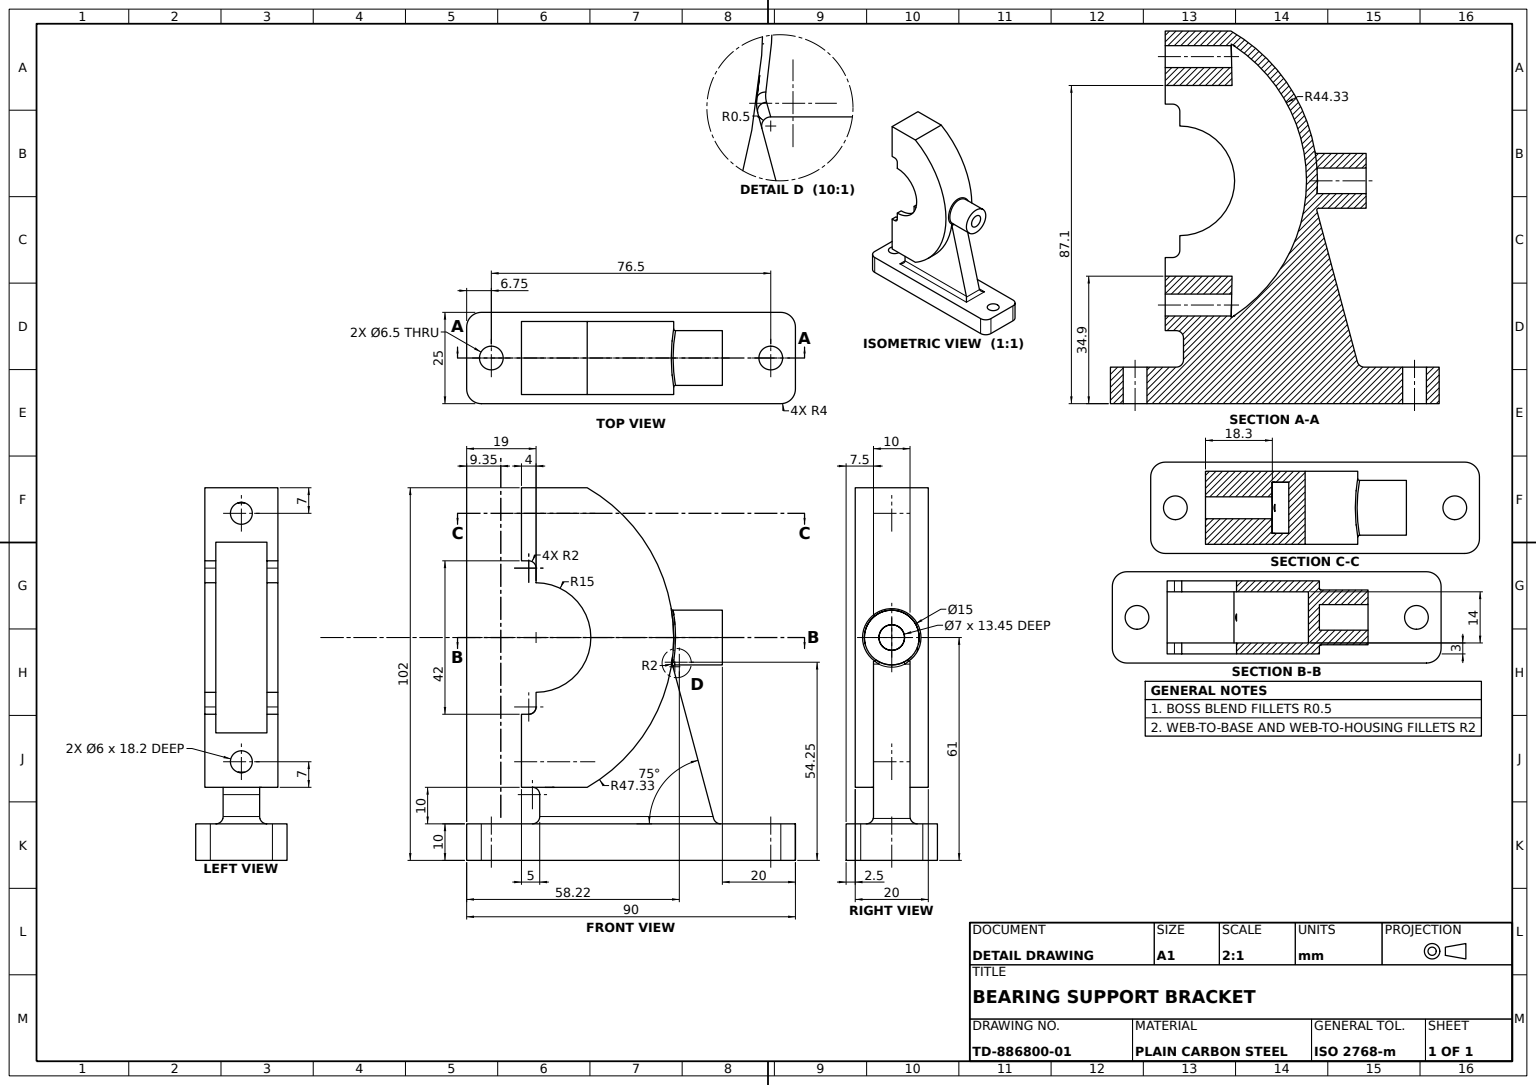
from build123d import *

# Parameters (mm, degrees)
BASE_PLATE_DEPTH              = 10
MOUNTING_HOLES_SKETCH_R       = 3.25
MOUNTING_HOLES_2X_6_5_DEPTH   = 10
UPRIGHT_WEB_SKETCH_W          = 48
UPRIGHT_WEB_SKETCH_H          = 12
UPRIGHT_WEB_DEPTH             = 30
UPRIGHT_WEB_TAPER             = 3
HOUSING_HALF_DEPTH            = 3
HOUSING_ARC_CUT_DEPTH         = 20
WEB_RELIEF_CUT_SKETCH_W       = 13.847905122
WEB_RELIEF_CUT_SKETCH_H       = 28.94973959
WEB_RELIEF_CUT_DEPTH          = 60
HOUSING_LUG_DEPTH             = 14
HOUSING_FLANGE_DEPTH          = 3
HOUSING_RIB_DEPTH             = 20
HOUSING_RELIEF_CUT_DEPTH      = 15
HOUSING_BODY_DEPTH            = 10
FILL_BLOCK_SKETCH_W           = 51.167533007
FILL_BLOCK_SKETCH_H           = 15.02058519
FILL_BLOCK_DEPTH              = 10
BEARING_SEAT_NOTCH_SKETCH_W   = 20.979401449
BEARING_SEAT_NOTCH_SKETCH_H   = 6.47797526
BEARING_SEAT_NOTCH_DEPTH      = 10
BASE_TO_HOUSING_FILLET_R2_R   = 2
SPLIT_BOLT_HOLES_SKETCH_R     = 3
SPLIT_BOLT_HOLES_DEPTH        = 19
FLANGE_FILLET_R2_R            = 2
HOUSING_EDGE_FILLET_R2_R      = 2
GREASE_NIPPLE_BOSS_SKETCH_R   = 7.5
GREASE_NIPPLE_BOSS_SKETCH_R_2 = 3.5
GREASE_NIPPLE_BOSS_DEPTH      = 15
GREASE_BOSS_FILLET_R0_5_R     = 0.5


with BuildPart() as part:
    # Base Plate Sketch → Base Plate (new body)
    with BuildSketch(Plane(origin=(0, 0, 0), x_dir=(1, 0, 0), z_dir=(0, 1, 0))):
        with BuildLine():
            Line((-41, 12.5), (41, 12.5))
            ThreePointArc((41, 12.5), (43.828427125, 11.328427125), (45, 8.5))
            Line((45, 8.5), (45, -8.5))
            ThreePointArc((45, -8.5), (43.828427125, -11.328427125), (41, -12.5))
            Line((41, -12.5), (-41, -12.5))
            ThreePointArc((-41, -12.5), (-43.828427125, -11.328427125), (-45, -8.5))
            Line((-45, -8.5), (-45, 8.5))
            ThreePointArc((-45, 8.5), (-43.828427125, 11.328427125), (-41, 12.5))
        make_face()
    extrude(amount=BASE_PLATE_DEPTH)

    # Mounting Holes Sketch → Mounting Holes 2xØ6.5 (cut)
    with BuildSketch(Plane(origin=(0, 10, 0), x_dir=(1, 0, 0), z_dir=(0, 1, 0))):
        with Locations(Location((-38.25, 0, 0), (0, 0, 270))):
            Circle(MOUNTING_HOLES_SKETCH_R)
        with Locations(Location((38.25, 0, 0), (0, 0, 270))):
            Circle(MOUNTING_HOLES_SKETCH_R)
    extrude(amount=-MOUNTING_HOLES_2X_6_5_DEPTH, mode=Mode.SUBTRACT)

    # Upright Web Sketch → Upright Web (add)
    with BuildSketch(Plane(origin=(0, 10, 0), x_dir=(1, 0, 0), z_dir=(0, 1, 0))):
        Rectangle(UPRIGHT_WEB_SKETCH_W, UPRIGHT_WEB_SKETCH_H)
    extrude(amount=UPRIGHT_WEB_DEPTH, taper=UPRIGHT_WEB_TAPER)

    # Housing Arc Cut Sketch → Housing Arc Cut (cut)
    with BuildSketch(Plane(origin=(0, 0, 7), x_dir=(-1, 0, 0), z_dir=(0, 0, -1))):
        with BuildLine():
            Line((12, 20), (30, 20))
            Line((30, 20), (30, 40))
            Line((30, 40), (-6.766315335, 40))
            ThreePointArc((-6.766315335, 40), (1.13659086, 28.611056704), (12, 20))
        make_face()
    extrude(amount=HOUSING_ARC_CUT_DEPTH, mode=Mode.SUBTRACT)

    # Web Relief Cut Sketch → Web Relief Cut (cut)
    with BuildSketch(Plane(origin=(-24.456905061, 1.281732082, 0), x_dir=(0, 0, 1), z_dir=(-0.998629534754574, 0.05233595624294398, 0))):
        with Locations((-0.74063995, 33.322014389)):
            Rectangle(WEB_RELIEF_CUT_SKETCH_W, WEB_RELIEF_CUT_SKETCH_H)
    extrude(amount=-WEB_RELIEF_CUT_DEPTH, mode=Mode.SUBTRACT)



with BuildPart() as body_2:
    # Housing Half Sketch → Housing Half (new body)
    with BuildSketch(Plane.XY.offset(10)):
        with BuildLine():
            Line((-26, 82), (-26, 76))
            ThreePointArc((-26, 76), (-11, 61), (-26, 46))
            Line((-26, 46), (-26, 40))
            Line((-26, 40), (-30, 40))
            Line((-30, 40), (-30, 20))
            Line((-30, 20), (-12, 20))
            ThreePointArc((-12, 20), (11.679663231, 61), (-12, 102))
            Line((-12, 102), (-30, 102))
            Line((-30, 102), (-30, 82))
            Line((-30, 82), (-26, 82))
        make_face()
    extrude(amount=-HOUSING_HALF_DEPTH)


with BuildPart() as part_1:
    add(part.part)

    add(body_2.part)  # Housing Lug merges body 2
    # Housing Lug Sketch → Housing Lug (add)
    with BuildSketch(Plane(origin=(0, 0, 7), x_dir=(-1, 0, 0), z_dir=(0, 0, -1))):
        with BuildLine():
            Line((30, 102), (12, 102))
            ThreePointArc((12, 102), (-11.679663231, 61), (12, 20))
            Line((12, 20), (30, 20))
            Line((30, 20), (30, 23))
            Line((30, 23), (12.817485057, 23))
            ThreePointArc((12.817485057, 23), (-8.679663231, 61), (12.817485057, 99))
            Line((12.817485057, 99), (30, 99))
            Line((30, 99), (30, 102))
        make_face()
    extrude(amount=HOUSING_LUG_DEPTH)

    # Housing Flange Sketch → Housing Flange (add)
    with BuildSketch(Plane(origin=(0, 0, -7), x_dir=(-1, 0, 0), z_dir=(0, 0, -1))):
        with BuildLine():
            Line((30, 102), (30, 82))
            Line((30, 82), (26, 82))
            Line((26, 82), (26, 76))
            ThreePointArc((26, 76), (11, 61), (26, 46))
            Line((26, 46), (26, 40))
            Line((26, 40), (30, 40))
            Line((30, 40), (30, 20))
            Line((30, 20), (12, 20))
            ThreePointArc((12, 20), (-11.679663231, 61), (12, 102))
            Line((12, 102), (30, 102))
        make_face()
    extrude(amount=HOUSING_FLANGE_DEPTH)

    # Housing Rib Sketch → Housing Rib (add)
    with BuildSketch(Plane.XY.offset(10)):
        Polygon((-30, 102), (-30, 87.099781417), (-11.701835925, 87.099781417), (-12, 102), align=None)
        Polygon((-30, 20), (-30, 34.9), (-11.701835925, 34.9), (-12, 20), align=None)
    extrude(amount=-HOUSING_RIB_DEPTH)

    # Housing Relief Cut Sketch → Housing Relief Cut (cut)
    with BuildSketch(Plane(origin=(0, 0.340975913, 6.506208002), x_dir=(1, 0, 0), z_dir=(0, 0.05233595624294398, 0.998629534754574))):
        Polygon((-24, 9.67227961), (24, 9.67227961), (23.599803921, 17.318955196), (-21.504261728, 19.68600307), (-23.475922207, 19.68600307), align=None)
        Polygon((-12.046627226, 19.68600307), (-21.504261728, 19.68600307), (23.599803921, 17.318955196), (24, 9.67227961), (26.480054023, 9.67227961), (26.480054023, 18.238066797), align=None)
        Polygon((-24, 9.67227961), (-23.475922207, 19.68600307), (-24.687478984, 19.68600307), (-24.687478984, 9.67227961), align=None)
    extrude(amount=-HOUSING_RELIEF_CUT_DEPTH, mode=Mode.SUBTRACT)


with BuildPart() as housing_relief_cut_piece_1:
    # of the separate pieces the step leaves, piece 1, a body of its own (housing_relief_cut_pieces)
    add(part_1.part.solids().sort_by_distance((-12, 102, -10))[0])



with BuildPart() as housing_relief_cut_piece_2:
    # of the separate pieces the step leaves, piece 2, a body of its own (housing_relief_cut_pieces)
    add(part_1.part.solids().sort_by_distance((-41, 10, -12.5))[0])


with BuildPart() as housing_relief_cut_piece_1_1:
    add(housing_relief_cut_piece_1.part)

    add(housing_relief_cut_piece_2.part)  # Housing Body merges Housing Relief Cut piece 2
    # Housing Body Sketch → Housing Body (add)
    with BuildSketch(Plane.XY.offset(5)):
        with BuildLine():
            Line((-27, 20), (-12, 20))
            ThreePointArc((-12, 20), (3.501198054, 34.403786208), (11.177379383, 54.12262082))
            Line((11.177379383, 54.12262082), (23, 10))
            Line((23, 10), (-25, 9.959503709))
            Line((-25, 9.959503709), (-25, 18))
            ThreePointArc((-25, 18), (-25.585786438, 19.414213562), (-27, 20))
        make_face()
    extrude(amount=-HOUSING_BODY_DEPTH)

    # Fill Block Sketch → Fill Block (add)
    with BuildSketch(Plane(origin=(0, 10, 0), x_dir=(1, 0, 0), z_dir=(0, 1, 0))):
        with Locations((0.896287519, 1.510292595)):
            Rectangle(FILL_BLOCK_SKETCH_W, FILL_BLOCK_SKETCH_H)
    extrude(amount=-FILL_BLOCK_DEPTH)

    # Bearing Seat Notch Sketch → Bearing Seat Notch (cut)
    with BuildSketch(Plane(origin=(0, 10, 0), x_dir=(1, 0, 0), z_dir=(0, 1, 0))):
        with Locations((-14.510299275, 8.23898763)):
            Rectangle(BEARING_SEAT_NOTCH_SKETCH_W, BEARING_SEAT_NOTCH_SKETCH_H)
    extrude(amount=BEARING_SEAT_NOTCH_DEPTH, mode=Mode.SUBTRACT)

    # Base To Housing Fillet R2
    base_to_housing_fillet_r2_edges = [housing_relief_cut_piece_1_1.edges().sort_by_distance(p)[0] for p in [
        (23, 10, 0),
        (-25, 10, 0),
        (-1, 10, 5),
        (-1, 10, -5),
    ]]
    fillet(base_to_housing_fillet_r2_edges, radius=BASE_TO_HOUSING_FILLET_R2_R)

    # Split Bolt Holes Sketch → Split Bolt Holes (cut)
    with BuildSketch(Plane.ZY.offset(30)):
        with Locations((0, 95)):
            Circle(SPLIT_BOLT_HOLES_SKETCH_R)
        with Locations((0, 27)):
            Circle(SPLIT_BOLT_HOLES_SKETCH_R)
    extrude(amount=-SPLIT_BOLT_HOLES_DEPTH, mode=Mode.SUBTRACT)

    # Flange Fillet R2
    flange_fillet_r2_edges = [housing_relief_cut_piece_1_1.edges().sort_by_distance(p)[0] for p in [
        (-26, 82, 8.5),
        (-26, 40, 8.5),
        (-26, 82, -8.5),
        (-26, 40, -8.5),
    ]]
    fillet(flange_fillet_r2_edges, radius=FLANGE_FILLET_R2_R)

    # Housing Edge Fillet R2
    housing_edge_fillet_r2_edges = [housing_relief_cut_piece_1_1.edges().sort_by_distance(p)[0] for p in [
        (11.177379383, 54.12262082, 0),
    ]]
    fillet(housing_edge_fillet_r2_edges, radius=HOUSING_EDGE_FILLET_R2_R)

    # Grease Nipple Boss Sketch → Grease Nipple Boss (add)
    with BuildSketch(Plane(origin=(25, 0, 0), x_dir=(0, 0, -1), z_dir=(1, 0, 0))):
        with Locations((0, 61)):
            Circle(GREASE_NIPPLE_BOSS_SKETCH_R)
        with Locations((0, 61)):
            Circle(GREASE_NIPPLE_BOSS_SKETCH_R_2, mode=Mode.SUBTRACT)
    extrude(amount=-GREASE_NIPPLE_BOSS_DEPTH)

    # Grease Boss Fillet R0.5
    grease_boss_fillet_r0_5_edges = [housing_relief_cut_piece_1_1.edges().sort_by_distance(p)[0] for p in [
        (11.224130168, 54.055042573, 2.831530734),
        (11.224130168, 54.055042573, -2.831530734),
        (11.344210129, 53.5, 0),
        (11.344210129, 53.5, 0),
    ]]
    fillet(grease_boss_fillet_r0_5_edges, radius=GREASE_BOSS_FILLET_R0_5_R)


solid = housing_relief_cut_piece_1_1.part
